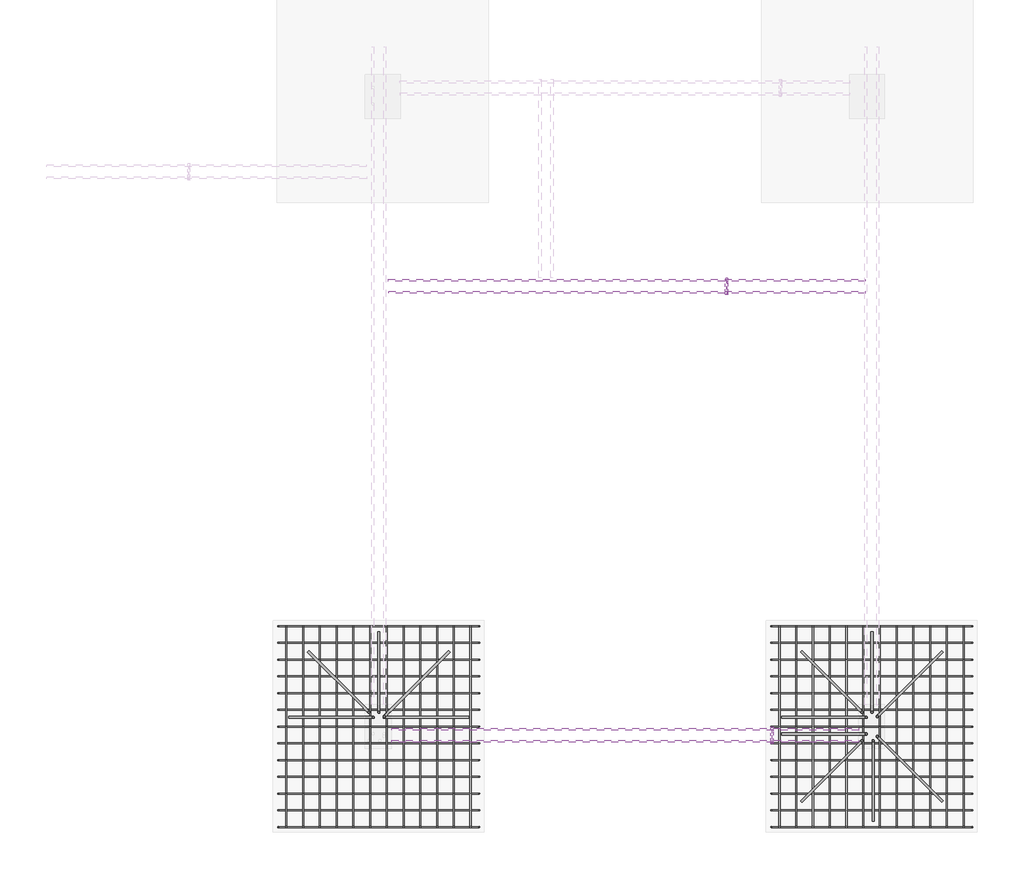
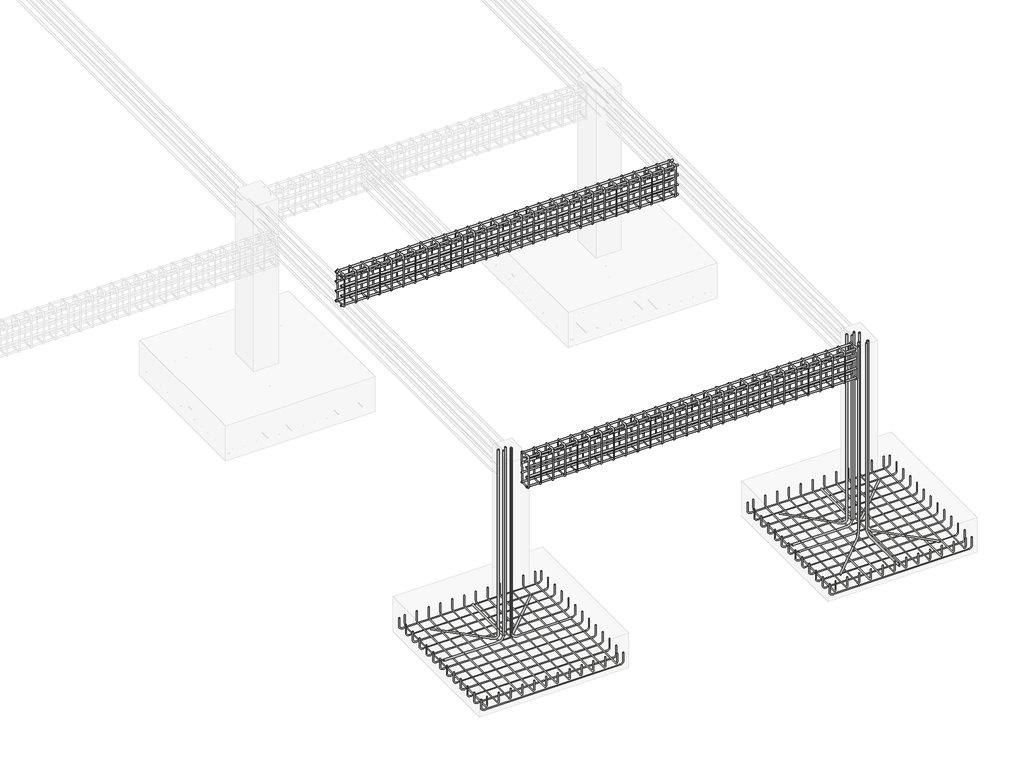
# One storey, part 3 of 10: 23 reinforcing bars.
"""IFC4 building model written with IfcOpenShell, lengths in millimetres."""

from ifc_helpers import new_model, si_unit, point, frame, origin, place, context, project, spatial, polyline, circle_curve, trimmed, segment, composite_curve, source, transform, mapped, element, save
from ifc_brep_helpers import swept_disk

model = new_model("IFC4")

# Units and contexts
model_context = context("Model", 3, world=origin())
ifc_project = project(units=[si_unit("LENGTHUNIT", "METRE", prefix="MILLI")], contexts=[model_context])

# Site, building, storey
site = spatial("IfcSite", under=ifc_project)
building = spatial("IfcBuilding", under=site)
storey = spatial("IfcBuildingStorey", under=building, Elevation=-2133.6)

# Reinforcing bars
placement = place(None, origin())
reinforcing_bar_shape = source(origin(), model_context, "Body", "SolidModel", [
    swept_disk(composite_curve([segment(polyline([(4240.1835638, -3095.8780823, -2393.6), (4240.1835638, -3095.8780823, -2504.1)]), True, "CONTINUOUS"), segment(trimmed(circle_curve(frame((4205.4335638, -3095.8780823, -2504.1), z_axis=(0.0, 1.0, 0.0), x_axis=(34.75, 0.0, 0.0)), 34.75), [point((4240.1835638, -3095.8780823, -2504.1))], [point((4205.4335638, -3095.8780823, -2538.85))], True, "CARTESIAN"), True, "CONTINUOUS"), segment(polyline([(4205.4335638, -3095.8780823, -2538.85), (2535.6335638, -3095.8780823, -2538.85)]), True, "CONTINUOUS"), segment(trimmed(circle_curve(frame((2535.6335638, -3095.8780823, -2504.1), z_axis=(0.0, 1.0, 0.0), x_axis=(0.0, 0.0, -34.75)), 34.75), [point((2535.6335638, -3095.8780823, -2538.85))], [point((2500.8835638, -3095.8780823, -2504.1))], True, "CARTESIAN"), True, "CONTINUOUS"), segment(polyline([(2500.8835638, -3095.8780823, -2504.1), (2500.8835638, -3095.8780823, -2393.6)]), True, "CONTINUOUS")], self_intersect=False), 4.75),
])
element("IfcReinforcingBar", 1, at=placement, inside=storey, context=model_context, shape_type="MappedRepresentation", body=[
    mapped(reinforcing_bar_shape, transform((0.0, 0.0, 0.0), x_axis=(1.0, 0.0, 0.0), y_axis=(0.0, 1.0, 0.0), z_axis=(0.0, 0.0, 1.0))),
    mapped(reinforcing_bar_shape, transform((0.0, -144.9416667, 0.0), x_axis=(1.0, 0.0, 0.0), y_axis=(0.0, 1.0, 0.0), z_axis=(0.0, 0.0, 1.0))),
    mapped(reinforcing_bar_shape, transform((0.0, -289.8833333, 0.0), x_axis=(1.0, 0.0, 0.0), y_axis=(0.0, 1.0, 0.0), z_axis=(0.0, 0.0, 1.0))),
    mapped(reinforcing_bar_shape, transform((0.0, -434.825, 0.0), x_axis=(1.0, 0.0, 0.0), y_axis=(0.0, 1.0, 0.0), z_axis=(0.0, 0.0, 1.0))),
    mapped(reinforcing_bar_shape, transform((0.0, -579.7666667, 0.0), x_axis=(1.0, 0.0, 0.0), y_axis=(0.0, 1.0, 0.0), z_axis=(0.0, 0.0, 1.0))),
    mapped(reinforcing_bar_shape, transform((0.0, -724.7083333, 0.0), x_axis=(1.0, 0.0, 0.0), y_axis=(0.0, 1.0, 0.0), z_axis=(0.0, 0.0, 1.0))),
    mapped(reinforcing_bar_shape, transform((0.0, -869.65, 0.0), x_axis=(1.0, 0.0, 0.0), y_axis=(0.0, 1.0, 0.0), z_axis=(0.0, 0.0, 1.0))),
    mapped(reinforcing_bar_shape, transform((0.0, -1014.5916667, 0.0), x_axis=(1.0, 0.0, 0.0), y_axis=(0.0, 1.0, 0.0), z_axis=(0.0, 0.0, 1.0))),
    mapped(reinforcing_bar_shape, transform((0.0, -1159.5333333, 0.0), x_axis=(1.0, 0.0, 0.0), y_axis=(0.0, 1.0, 0.0), z_axis=(0.0, 0.0, 1.0))),
    mapped(reinforcing_bar_shape, transform((0.0, -1304.475, 0.0), x_axis=(1.0, 0.0, 0.0), y_axis=(0.0, 1.0, 0.0), z_axis=(0.0, 0.0, 1.0))),
    mapped(reinforcing_bar_shape, transform((0.0, -1449.4166667, 0.0), x_axis=(1.0, 0.0, 0.0), y_axis=(0.0, 1.0, 0.0), z_axis=(0.0, 0.0, 1.0))),
    mapped(reinforcing_bar_shape, transform((0.0, -1594.3583333, 0.0), x_axis=(1.0, 0.0, 0.0), y_axis=(0.0, 1.0, 0.0), z_axis=(0.0, 0.0, 1.0))),
    mapped(reinforcing_bar_shape, transform((0.0, -1739.3, 0.0), x_axis=(1.0, 0.0, 0.0), y_axis=(0.0, 1.0, 0.0), z_axis=(0.0, 0.0, 1.0))),
])
reinforcing_bar_2_shape = source(origin(), model_context, "Body", "SolidModel", [
    swept_disk(composite_curve([segment(polyline([(4165.2256133, -4835.1780823, -2379.223371), (4165.2256133, -4835.1780823, -2489.723371)]), True, "CONTINUOUS"), segment(trimmed(circle_curve(frame((4165.2256133, -4800.4280823, -2489.723371), z_axis=(1.0, 0.0, 0.0), x_axis=(0.0, -34.75, 0.0)), 34.75), [point((4165.2256133, -4835.1780823, -2489.723371))], [point((4165.2256133, -4800.4280823, -2524.473371))], True, "CARTESIAN"), True, "CONTINUOUS"), segment(polyline([(4165.2256133, -4800.4280823, -2524.473371), (4165.2256133, -3130.6280823, -2524.473371)]), True, "CONTINUOUS"), segment(trimmed(circle_curve(frame((4165.2256133, -3130.6280823, -2489.723371), z_axis=(1.0, 0.0, 0.0), x_axis=(0.0, 0.0, -34.75)), 34.75), [point((4165.2256133, -3130.6280823, -2524.473371))], [point((4165.2256133, -3095.8780823, -2489.723371))], True, "CARTESIAN"), True, "CONTINUOUS"), segment(polyline([(4165.2256133, -3095.8780823, -2489.723371), (4165.2256133, -3095.8780823, -2379.223371)]), True, "CONTINUOUS")], self_intersect=False), 4.75),
])
element("IfcReinforcingBar", 2, at=placement, inside=storey, context=model_context, shape_type="MappedRepresentation", body=[
    mapped(reinforcing_bar_2_shape, transform((0.0, 0.0, 0.0), x_axis=(1.0, 0.0, 0.0), y_axis=(0.0, 1.0, 0.0), z_axis=(0.0, 0.0, 1.0))),
    mapped(reinforcing_bar_2_shape, transform((-144.8323389, 0.0, 0.0), x_axis=(1.0, 0.0, 0.0), y_axis=(0.0, 1.0, 0.0), z_axis=(0.0, 0.0, 1.0))),
    mapped(reinforcing_bar_2_shape, transform((-289.6646779, 0.0, 0.0), x_axis=(1.0, 0.0, 0.0), y_axis=(0.0, 1.0, 0.0), z_axis=(0.0, 0.0, 1.0))),
    mapped(reinforcing_bar_2_shape, transform((-434.4970168, 0.0, 0.0), x_axis=(1.0, 0.0, 0.0), y_axis=(0.0, 1.0, 0.0), z_axis=(0.0, 0.0, 1.0))),
    mapped(reinforcing_bar_2_shape, transform((-579.3293558, 0.0, 0.0), x_axis=(1.0, 0.0, 0.0), y_axis=(0.0, 1.0, 0.0), z_axis=(0.0, 0.0, 1.0))),
    mapped(reinforcing_bar_2_shape, transform((-724.1616947, 0.0, 0.0), x_axis=(1.0, 0.0, 0.0), y_axis=(0.0, 1.0, 0.0), z_axis=(0.0, 0.0, 1.0))),
    mapped(reinforcing_bar_2_shape, transform((-868.9940337, 0.0, 0.0), x_axis=(1.0, 0.0, 0.0), y_axis=(0.0, 1.0, 0.0), z_axis=(0.0, 0.0, 1.0))),
    mapped(reinforcing_bar_2_shape, transform((-1013.8263726, 0.0, 0.0), x_axis=(1.0, 0.0, 0.0), y_axis=(0.0, 1.0, 0.0), z_axis=(0.0, 0.0, 1.0))),
    mapped(reinforcing_bar_2_shape, transform((-1158.6587116, 0.0, 0.0), x_axis=(1.0, 0.0, 0.0), y_axis=(0.0, 1.0, 0.0), z_axis=(0.0, 0.0, 1.0))),
    mapped(reinforcing_bar_2_shape, transform((-1303.4910505, 0.0, 0.0), x_axis=(1.0, 0.0, 0.0), y_axis=(0.0, 1.0, 0.0), z_axis=(0.0, 0.0, 1.0))),
    mapped(reinforcing_bar_2_shape, transform((-1448.3233895, 0.0, 0.0), x_axis=(1.0, 0.0, 0.0), y_axis=(0.0, 1.0, 0.0), z_axis=(0.0, 0.0, 1.0))),
    mapped(reinforcing_bar_2_shape, transform((-1593.1557284, 0.0, 0.0), x_axis=(1.0, 0.0, 0.0), y_axis=(0.0, 1.0, 0.0), z_axis=(0.0, 0.0, 1.0))),
])
reinforcing_bar_3_shape = source(origin(), model_context, "Body", "SolidModel", [
    swept_disk(composite_curve([segment(polyline([(8507.3835638, -3095.8780823, -2393.6), (8507.3835638, -3095.8780823, -2504.1)]), True, "CONTINUOUS"), segment(trimmed(circle_curve(frame((8472.6335638, -3095.8780823, -2504.1), z_axis=(0.0, 1.0, 0.0), x_axis=(34.75, 0.0, 0.0)), 34.75), [point((8507.3835638, -3095.8780823, -2504.1))], [point((8472.6335638, -3095.8780823, -2538.85))], True, "CARTESIAN"), True, "CONTINUOUS"), segment(polyline([(8472.6335638, -3095.8780823, -2538.85), (6802.8335638, -3095.8780823, -2538.85)]), True, "CONTINUOUS"), segment(trimmed(circle_curve(frame((6802.8335638, -3095.8780823, -2504.1), z_axis=(0.0, 1.0, 0.0), x_axis=(0.0, 0.0, -34.75)), 34.75), [point((6802.8335638, -3095.8780823, -2538.85))], [point((6768.0835638, -3095.8780823, -2504.1))], True, "CARTESIAN"), True, "CONTINUOUS"), segment(polyline([(6768.0835638, -3095.8780823, -2504.1), (6768.0835638, -3095.8780823, -2393.6)]), True, "CONTINUOUS")], self_intersect=False), 4.75),
])
element("IfcReinforcingBar", 3, at=placement, inside=storey, context=model_context, shape_type="MappedRepresentation", body=[
    mapped(reinforcing_bar_3_shape, transform((0.0, 0.0, 0.0), x_axis=(1.0, 0.0, 0.0), y_axis=(0.0, 1.0, 0.0), z_axis=(0.0, 0.0, 1.0))),
    mapped(reinforcing_bar_3_shape, transform((0.0, -144.9416667, 0.0), x_axis=(1.0, 0.0, 0.0), y_axis=(0.0, 1.0, 0.0), z_axis=(0.0, 0.0, 1.0))),
    mapped(reinforcing_bar_3_shape, transform((0.0, -289.8833333, 0.0), x_axis=(1.0, 0.0, 0.0), y_axis=(0.0, 1.0, 0.0), z_axis=(0.0, 0.0, 1.0))),
    mapped(reinforcing_bar_3_shape, transform((0.0, -434.825, 0.0), x_axis=(1.0, 0.0, 0.0), y_axis=(0.0, 1.0, 0.0), z_axis=(0.0, 0.0, 1.0))),
    mapped(reinforcing_bar_3_shape, transform((0.0, -579.7666667, 0.0), x_axis=(1.0, 0.0, 0.0), y_axis=(0.0, 1.0, 0.0), z_axis=(0.0, 0.0, 1.0))),
    mapped(reinforcing_bar_3_shape, transform((0.0, -724.7083333, 0.0), x_axis=(1.0, 0.0, 0.0), y_axis=(0.0, 1.0, 0.0), z_axis=(0.0, 0.0, 1.0))),
    mapped(reinforcing_bar_3_shape, transform((0.0, -869.65, 0.0), x_axis=(1.0, 0.0, 0.0), y_axis=(0.0, 1.0, 0.0), z_axis=(0.0, 0.0, 1.0))),
    mapped(reinforcing_bar_3_shape, transform((0.0, -1014.5916667, 0.0), x_axis=(1.0, 0.0, 0.0), y_axis=(0.0, 1.0, 0.0), z_axis=(0.0, 0.0, 1.0))),
    mapped(reinforcing_bar_3_shape, transform((0.0, -1159.5333333, 0.0), x_axis=(1.0, 0.0, 0.0), y_axis=(0.0, 1.0, 0.0), z_axis=(0.0, 0.0, 1.0))),
    mapped(reinforcing_bar_3_shape, transform((0.0, -1304.475, 0.0), x_axis=(1.0, 0.0, 0.0), y_axis=(0.0, 1.0, 0.0), z_axis=(0.0, 0.0, 1.0))),
    mapped(reinforcing_bar_3_shape, transform((0.0, -1449.4166667, 0.0), x_axis=(1.0, 0.0, 0.0), y_axis=(0.0, 1.0, 0.0), z_axis=(0.0, 0.0, 1.0))),
    mapped(reinforcing_bar_3_shape, transform((0.0, -1594.3583333, 0.0), x_axis=(1.0, 0.0, 0.0), y_axis=(0.0, 1.0, 0.0), z_axis=(0.0, 0.0, 1.0))),
    mapped(reinforcing_bar_3_shape, transform((0.0, -1739.3, 0.0), x_axis=(1.0, 0.0, 0.0), y_axis=(0.0, 1.0, 0.0), z_axis=(0.0, 0.0, 1.0))),
])
reinforcing_bar_4_shape = source(origin(), model_context, "Body", "SolidModel", [
    swept_disk(composite_curve([segment(polyline([(8432.4256133, -4835.1780823, -2379.223371), (8432.4256133, -4835.1780823, -2489.723371)]), True, "CONTINUOUS"), segment(trimmed(circle_curve(frame((8432.4256133, -4800.4280823, -2489.723371), z_axis=(1.0, 0.0, 0.0), x_axis=(0.0, -34.75, 0.0)), 34.75), [point((8432.4256133, -4835.1780823, -2489.723371))], [point((8432.4256133, -4800.4280823, -2524.473371))], True, "CARTESIAN"), True, "CONTINUOUS"), segment(polyline([(8432.4256133, -4800.4280823, -2524.473371), (8432.4256133, -3130.6280823, -2524.473371)]), True, "CONTINUOUS"), segment(trimmed(circle_curve(frame((8432.4256133, -3130.6280823, -2489.723371), z_axis=(1.0, 0.0, 0.0), x_axis=(0.0, 0.0, -34.75)), 34.75), [point((8432.4256133, -3130.6280823, -2524.473371))], [point((8432.4256133, -3095.8780823, -2489.723371))], True, "CARTESIAN"), True, "CONTINUOUS"), segment(polyline([(8432.4256133, -3095.8780823, -2489.723371), (8432.4256133, -3095.8780823, -2379.223371)]), True, "CONTINUOUS")], self_intersect=False), 4.75),
])
element("IfcReinforcingBar", 4, at=placement, inside=storey, context=model_context, shape_type="MappedRepresentation", body=[
    mapped(reinforcing_bar_4_shape, transform((0.0, 0.0, 0.0), x_axis=(1.0, 0.0, 0.0), y_axis=(0.0, 1.0, 0.0), z_axis=(0.0, 0.0, 1.0))),
    mapped(reinforcing_bar_4_shape, transform((-144.8323389, 0.0, 0.0), x_axis=(1.0, 0.0, 0.0), y_axis=(0.0, 1.0, 0.0), z_axis=(0.0, 0.0, 1.0))),
    mapped(reinforcing_bar_4_shape, transform((-289.6646779, 0.0, 0.0), x_axis=(1.0, 0.0, 0.0), y_axis=(0.0, 1.0, 0.0), z_axis=(0.0, 0.0, 1.0))),
    mapped(reinforcing_bar_4_shape, transform((-434.4970168, 0.0, 0.0), x_axis=(1.0, 0.0, 0.0), y_axis=(0.0, 1.0, 0.0), z_axis=(0.0, 0.0, 1.0))),
    mapped(reinforcing_bar_4_shape, transform((-579.3293558, 0.0, 0.0), x_axis=(1.0, 0.0, 0.0), y_axis=(0.0, 1.0, 0.0), z_axis=(0.0, 0.0, 1.0))),
    mapped(reinforcing_bar_4_shape, transform((-724.1616947, 0.0, 0.0), x_axis=(1.0, 0.0, 0.0), y_axis=(0.0, 1.0, 0.0), z_axis=(0.0, 0.0, 1.0))),
    mapped(reinforcing_bar_4_shape, transform((-868.9940337, 0.0, 0.0), x_axis=(1.0, 0.0, 0.0), y_axis=(0.0, 1.0, 0.0), z_axis=(0.0, 0.0, 1.0))),
    mapped(reinforcing_bar_4_shape, transform((-1013.8263726, 0.0, 0.0), x_axis=(1.0, 0.0, 0.0), y_axis=(0.0, 1.0, 0.0), z_axis=(0.0, 0.0, 1.0))),
    mapped(reinforcing_bar_4_shape, transform((-1158.6587116, 0.0, 0.0), x_axis=(1.0, 0.0, 0.0), y_axis=(0.0, 1.0, 0.0), z_axis=(0.0, 0.0, 1.0))),
    mapped(reinforcing_bar_4_shape, transform((-1303.4910505, 0.0, 0.0), x_axis=(1.0, 0.0, 0.0), y_axis=(0.0, 1.0, 0.0), z_axis=(0.0, 0.0, 1.0))),
    mapped(reinforcing_bar_4_shape, transform((-1448.3233895, 0.0, 0.0), x_axis=(1.0, 0.0, 0.0), y_axis=(0.0, 1.0, 0.0), z_axis=(0.0, 0.0, 1.0))),
    mapped(reinforcing_bar_4_shape, transform((-1593.1557284, 0.0, 0.0), x_axis=(1.0, 0.0, 0.0), y_axis=(0.0, 1.0, 0.0), z_axis=(0.0, 0.0, 1.0))),
])
element("IfcReinforcingBar", 5, at=placement, inside=storey, context=model_context, shape_type="SolidModel", body=[
    swept_disk(composite_curve([segment(polyline([(7552.4335638, -3841.2447039, -40.0), (7552.4335638, -3841.2447039, -2426.55)]), True, "CONTINUOUS"), segment(trimmed(circle_curve(frame((7505.0220542, -3793.8331942, -2426.55), z_axis=(0.7071067811865519, 0.7071067811865431, 0.0), x_axis=(47.4115096000005, -47.4115096999999, 0.0)), 67.05), [point((7552.4335638, -3841.2447039, -2426.55))], [point((7505.0220542, -3793.8331942, -2493.6))], True, "CARTESIAN"), True, "CONTINUOUS"), segment(polyline([(7505.0220542, -3793.8331942, -2493.6), (7028.0116308, -3316.8227708, -2493.6)]), True, "CONTINUOUS")], self_intersect=False), 9.55),
])
element("IfcReinforcingBar", 6, at=placement, inside=storey, context=model_context, shape_type="SolidModel", body=[
    swept_disk(composite_curve([segment(polyline([(7686.0335638, -3879.3447039, -40.0), (7686.0335638, -3879.3447039, -2426.55)]), True, "CONTINUOUS"), segment(trimmed(circle_curve(frame((7733.4450735, -3831.9331942, -2426.55), z_axis=(0.7071067811865519, -0.7071067811865431, 0.0), x_axis=(-47.41150970000035, -47.4115096999999, 0.0)), 67.05), [point((7686.0335638, -3879.3447039, -2426.55))], [point((7733.4450735, -3831.9331942, -2493.6))], True, "CARTESIAN"), True, "CONTINUOUS"), segment(polyline([(7733.4450735, -3831.9331942, -2493.6), (8248.5554969, -3316.8227708, -2493.6)]), True, "CONTINUOUS")], self_intersect=False), 9.55),
])
element("IfcReinforcingBar", 7, at=placement, inside=storey, context=model_context, shape_type="SolidModel", body=[
    swept_disk(composite_curve([segment(polyline([(7552.4335638, -4089.8114607, -40.0), (7552.4335638, -4089.8114607, -2426.55)]), True, "CONTINUOUS"), segment(trimmed(circle_curve(frame((7505.0220542, -4137.2229704, -2426.55), z_axis=(-0.7071067811865519, 0.7071067811865431, 0.0), x_axis=(47.4115096000005, 47.4115096999999, 0.0)), 67.05), [point((7552.4335638, -4089.8114607, -2426.55))], [point((7505.0220542, -4137.2229704, -2493.6))], True, "CARTESIAN"), True, "CONTINUOUS"), segment(polyline([(7505.0220542, -4137.2229704, -2493.6), (7028.0116308, -4614.2333938, -2493.6)]), True, "CONTINUOUS")], self_intersect=False), 9.55),
])
element("IfcReinforcingBar", 8, at=placement, inside=storey, context=model_context, shape_type="SolidModel", body=[
    swept_disk(composite_curve([segment(polyline([(7686.0335638, -4051.7114607, -40.0), (7686.0335638, -4051.7114607, -2426.55)]), True, "CONTINUOUS"), segment(trimmed(circle_curve(frame((7733.4450735, -4099.1229704, -2426.55), z_axis=(-0.7071067811865519, -0.7071067811865431, 0.0), x_axis=(-47.41150970000035, 47.4115096999999, 0.0)), 67.05), [point((7686.0335638, -4051.7114607, -2426.55))], [point((7733.4450735, -4099.1229704, -2493.6))], True, "CARTESIAN"), True, "CONTINUOUS"), segment(polyline([(7733.4450735, -4099.1229704, -2493.6), (8248.5554969, -4614.2333938, -2493.6)]), True, "CONTINUOUS")], self_intersect=False), 9.55),
])
element("IfcReinforcingBar", 9, at=placement, inside=storey, context=model_context, shape_type="SolidModel", body=[
    swept_disk(composite_curve([segment(polyline([(7639.4194855, -3841.2447039, -40.0), (7639.4194855, -3841.2447039, -2426.55)]), True, "CONTINUOUS"), segment(trimmed(circle_curve(frame((7639.4194855, -3774.1947039, -2426.55), z_axis=(1.0, 0.0, 0.0), x_axis=(0.0, -67.04999999999973, 0.0)), 67.05), [point((7639.4194855, -3841.2447039, -2426.55))], [point((7639.4194855, -3774.1947039, -2493.6))], True, "CARTESIAN"), True, "CONTINUOUS"), segment(polyline([(7639.4194855, -3774.1947039, -2493.6), (7639.4194855, -3146.9447039, -2493.6)]), True, "CONTINUOUS")], self_intersect=False), 9.55),
])
element("IfcReinforcingBar", 10, at=placement, inside=storey, context=model_context, shape_type="SolidModel", body=[
    swept_disk(composite_curve([segment(polyline([(7649.4194855, -4089.8114607, -40.0), (7649.4194855, -4089.8114607, -2426.55)]), True, "CONTINUOUS"), segment(trimmed(circle_curve(frame((7649.4194855, -4156.8614607, -2426.55), z_axis=(-1.0, 0.0, 0.0), x_axis=(0.0, 67.04999999999973, 0.0)), 67.05), [point((7649.4194855, -4089.8114607, -2426.55))], [point((7649.4194855, -4156.8614607, -2493.6))], True, "CARTESIAN"), True, "CONTINUOUS"), segment(polyline([(7649.4194855, -4156.8614607, -2493.6), (7649.4194855, -4784.1114607, -2493.6)]), True, "CONTINUOUS")], self_intersect=False), 9.55),
])
element("IfcReinforcingBar", 11, at=placement, inside=storey, context=model_context, shape_type="SolidModel", body=[
    swept_disk(composite_curve([segment(polyline([(7590.5335638, -3886.2447039, -40.0), (7590.5335638, -3886.2447039, -2426.55)]), True, "CONTINUOUS"), segment(trimmed(circle_curve(frame((7523.4835638, -3886.2447039, -2426.55), z_axis=(0.0, 1.0, 0.0), x_axis=(67.04999999999927, 0.0, 0.0)), 67.05), [point((7590.5335638, -3886.2447039, -2426.55))], [point((7523.4835638, -3886.2447039, -2493.6))], True, "CARTESIAN"), True, "CONTINUOUS"), segment(polyline([(7523.4835638, -3886.2447039, -2493.6), (6858.1335638, -3886.2447039, -2493.6)]), True, "CONTINUOUS")], self_intersect=False), 9.55),
])
element("IfcReinforcingBar", 12, at=placement, inside=storey, context=model_context, shape_type="SolidModel", body=[
    swept_disk(composite_curve([segment(polyline([(7590.5335638, -4029.5829002, -40.0), (7590.5335638, -4029.5829002, -2426.55)]), True, "CONTINUOUS"), segment(trimmed(circle_curve(frame((7523.4835638, -4029.5829002, -2426.55), z_axis=(0.0, 1.0, 0.0), x_axis=(67.04999999999927, 0.0, 0.0)), 67.05), [point((7590.5335638, -4029.5829002, -2426.55))], [point((7523.4835638, -4029.5829002, -2493.6))], True, "CARTESIAN"), True, "CONTINUOUS"), segment(polyline([(7523.4835638, -4029.5829002, -2493.6), (6858.1335638, -4029.5829002, -2493.6)]), True, "CONTINUOUS")], self_intersect=False), 9.55),
])
element("IfcReinforcingBar", 13, at=placement, inside=storey, context=model_context, shape_type="SolidModel", body=[
    swept_disk(composite_curve([segment(polyline([(3285.2335638, -3841.2447039, -40.0), (3285.2335638, -3841.2447039, -2426.55)]), True, "CONTINUOUS"), segment(trimmed(circle_curve(frame((3237.8220542, -3793.8331942, -2426.55), z_axis=(0.7071067811865519, 0.7071067811865431, 0.0), x_axis=(47.411509600000045, -47.4115096999999, 0.0)), 67.05), [point((3285.2335638, -3841.2447039, -2426.55))], [point((3237.8220542, -3793.8331942, -2493.6))], True, "CARTESIAN"), True, "CONTINUOUS"), segment(polyline([(3237.8220542, -3793.8331942, -2493.6), (2760.8116308, -3316.8227708, -2493.6)]), True, "CONTINUOUS")], self_intersect=False), 9.55),
])
element("IfcReinforcingBar", 14, at=placement, inside=storey, context=model_context, shape_type="SolidModel", body=[
    swept_disk(composite_curve([segment(polyline([(3418.8335638, -3879.3447039, -40.0), (3418.8335638, -3879.3447039, -2426.55)]), True, "CONTINUOUS"), segment(trimmed(circle_curve(frame((3466.2450735, -3831.9331942, -2426.55), z_axis=(0.7071067811865519, -0.7071067811865431, 0.0), x_axis=(-47.41150970000035, -47.4115096999999, 0.0)), 67.05), [point((3418.8335638, -3879.3447039, -2426.55))], [point((3466.2450735, -3831.9331942, -2493.6))], True, "CARTESIAN"), True, "CONTINUOUS"), segment(polyline([(3466.2450735, -3831.9331942, -2493.6), (3981.3554969, -3316.8227708, -2493.6)]), True, "CONTINUOUS")], self_intersect=False), 9.55),
])
element("IfcReinforcingBar", 15, at=placement, inside=storey, context=model_context, shape_type="SolidModel", body=[
    swept_disk(composite_curve([segment(polyline([(3372.2194855, -3841.2447039, -40.0), (3372.2194855, -3841.2447039, -2426.55)]), True, "CONTINUOUS"), segment(trimmed(circle_curve(frame((3372.2194855, -3774.1947039, -2426.55), z_axis=(1.0, 0.0, 0.0), x_axis=(0.0, -67.04999999999973, 0.0)), 67.05), [point((3372.2194855, -3841.2447039, -2426.55))], [point((3372.2194855, -3774.1947039, -2493.6))], True, "CARTESIAN"), True, "CONTINUOUS"), segment(polyline([(3372.2194855, -3774.1947039, -2493.6), (3372.2194855, -3146.9447039, -2493.6)]), True, "CONTINUOUS")], self_intersect=False), 9.55),
])
element("IfcReinforcingBar", 16, at=placement, inside=storey, context=model_context, shape_type="SolidModel", body=[
    swept_disk(composite_curve([segment(polyline([(3323.3335638, -3886.2447039, -40.0), (3323.3335638, -3886.2447039, -2426.55)]), True, "CONTINUOUS"), segment(trimmed(circle_curve(frame((3256.2835638, -3886.2447039, -2426.55), z_axis=(0.0, 1.0, 0.0), x_axis=(67.04999999999973, 0.0, 0.0)), 67.05), [point((3323.3335638, -3886.2447039, -2426.55))], [point((3256.2835638, -3886.2447039, -2493.6))], True, "CARTESIAN"), True, "CONTINUOUS"), segment(polyline([(3256.2835638, -3886.2447039, -2493.6), (2590.9335638, -3886.2447039, -2493.6)]), True, "CONTINUOUS")], self_intersect=False), 9.55),
])
element("IfcReinforcingBar", 17, at=placement, inside=storey, context=model_context, shape_type="SolidModel", body=[
    swept_disk(composite_curve([segment(polyline([(3418.8335638, -3886.2447039, -40.0), (3418.8335638, -3886.2447039, -2426.55)]), True, "CONTINUOUS"), segment(trimmed(circle_curve(frame((3485.8835638, -3886.2447039, -2426.55), z_axis=(0.0, -1.0, 0.0), x_axis=(-67.05000000000018, 0.0, 0.0)), 67.05), [point((3418.8335638, -3886.2447039, -2426.55))], [point((3485.8835638, -3886.2447039, -2493.6))], True, "CARTESIAN"), True, "CONTINUOUS"), segment(polyline([(3485.8835638, -3886.2447039, -2493.6), (4151.2335638, -3886.2447039, -2493.6)]), True, "CONTINUOUS")], self_intersect=False), 9.55),
])
reinforcing_bar_5_shape = source(origin(), model_context, "Body", "SolidModel", [
    swept_disk(composite_curve([segment(polyline([(3502.9475179, -4011.6213007, -109.4049959), (3502.9475179, -4069.0271895, -51.9991072)]), True, "CONTINUOUS"), segment(trimmed(circle_curve(frame((3502.9475179, -4086.5280823, -69.5), z_axis=(1.0, 0.0, 0.0), x_axis=(0.0, 17.500892799999747, 17.500892800000003)), 24.75), [point((3502.9475179, -4069.0271895, -51.9991072))], [point((3502.9475179, -4111.2780823, -69.5))], True, "CARTESIAN"), True, "CONTINUOUS"), segment(polyline([(3502.9475179, -4111.2780823, -69.5), (3502.9475179, -4111.2780823, -430.5)]), True, "CONTINUOUS"), segment(trimmed(circle_curve(frame((3502.9475179, -4086.5280823, -430.5), z_axis=(1.0, 0.0, 0.0), x_axis=(0.0, -24.750000000000455, 0.0)), 24.75), [point((3502.9475179, -4111.2780823, -430.5))], [point((3502.9475179, -4086.5280823, -455.25))], True, "CARTESIAN"), True, "CONTINUOUS"), segment(polyline([(3502.9475179, -4086.5280823, -455.25), (3502.9475179, -3996.9280823, -455.25)]), True, "CONTINUOUS"), segment(trimmed(circle_curve(frame((3502.3748941, -3996.9280823, -430.5066251), z_axis=(0.9997323196529888, 0.0, 0.02313631434032496), x_axis=(0.5726238000002013, 0.0, -24.743374899999992)), 24.75), [point((3502.9475179, -3996.9280823, -455.25))], [point((3502.3748941, -3972.1780823, -430.5066251))], True, "CARTESIAN"), True, "CONTINUOUS"), segment(polyline([(3502.3748941, -3972.1780823, -430.5066251), (3494.0201417, -3972.1780823, -69.4933749)]), True, "CONTINUOUS"), segment(trimmed(circle_curve(frame((3494.0201417, -3996.9280823, -69.4933749), z_axis=(0.9997323196529888, 0.0, 0.02313631434032496), x_axis=(0.0, 24.75, 0.0)), 24.75), [point((3494.0201417, -3972.1780823, -69.4933749))], [point((3493.4475179, -3996.9280823, -44.75))], True, "CARTESIAN"), True, "CONTINUOUS"), segment(polyline([(3493.4475179, -3996.9280823, -44.75), (3493.4475179, -4086.5280823, -44.75)]), True, "CONTINUOUS"), segment(trimmed(circle_curve(frame((3493.4475179, -4086.5280823, -69.5), z_axis=(1.0, 0.0, 0.0), x_axis=(0.0, 0.0, 24.75)), 24.75), [point((3493.4475179, -4086.5280823, -44.75))], [point((3493.4475179, -4104.0289751, -87.0008928))], True, "CARTESIAN"), True, "CONTINUOUS"), segment(polyline([(3493.4475179, -4104.0289751, -87.0008928), (3493.4475179, -4046.6230864, -144.4067815)]), True, "CONTINUOUS")], self_intersect=False), 4.75),
])
element("IfcReinforcingBar", 18, at=placement, inside=storey, context=model_context, shape_type="MappedRepresentation", body=[
    mapped(reinforcing_bar_5_shape, transform((0.0, 0.0, 0.0), x_axis=(1.0, 0.0, 0.0), y_axis=(0.0, 1.0, 0.0), z_axis=(0.0, 0.0, 1.0))),
    mapped(reinforcing_bar_5_shape, transform((148.9068906, 0.0, 0.0), x_axis=(1.0, 0.0, 0.0), y_axis=(0.0, 1.0, 0.0), z_axis=(0.0, 0.0, 1.0))),
    mapped(reinforcing_bar_5_shape, transform((297.8137812, 0.0, 0.0), x_axis=(1.0, 0.0, 0.0), y_axis=(0.0, 1.0, 0.0), z_axis=(0.0, 0.0, 1.0))),
    mapped(reinforcing_bar_5_shape, transform((446.7206718, 0.0, 0.0), x_axis=(1.0, 0.0, 0.0), y_axis=(0.0, 1.0, 0.0), z_axis=(0.0, 0.0, 1.0))),
    mapped(reinforcing_bar_5_shape, transform((595.6275624, 0.0, 0.0), x_axis=(1.0, 0.0, 0.0), y_axis=(0.0, 1.0, 0.0), z_axis=(0.0, 0.0, 1.0))),
    mapped(reinforcing_bar_5_shape, transform((744.5344529, 0.0, 0.0), x_axis=(1.0, 0.0, 0.0), y_axis=(0.0, 1.0, 0.0), z_axis=(0.0, 0.0, 1.0))),
    mapped(reinforcing_bar_5_shape, transform((893.4413435, 0.0, 0.0), x_axis=(1.0, 0.0, 0.0), y_axis=(0.0, 1.0, 0.0), z_axis=(0.0, 0.0, 1.0))),
    mapped(reinforcing_bar_5_shape, transform((1042.3482341, 0.0, 0.0), x_axis=(1.0, 0.0, 0.0), y_axis=(0.0, 1.0, 0.0), z_axis=(0.0, 0.0, 1.0))),
    mapped(reinforcing_bar_5_shape, transform((1191.2551247, 0.0, 0.0), x_axis=(1.0, 0.0, 0.0), y_axis=(0.0, 1.0, 0.0), z_axis=(0.0, 0.0, 1.0))),
    mapped(reinforcing_bar_5_shape, transform((1340.1620153, 0.0, 0.0), x_axis=(1.0, 0.0, 0.0), y_axis=(0.0, 1.0, 0.0), z_axis=(0.0, 0.0, 1.0))),
    mapped(reinforcing_bar_5_shape, transform((1489.0689059, 0.0, 0.0), x_axis=(1.0, 0.0, 0.0), y_axis=(0.0, 1.0, 0.0), z_axis=(0.0, 0.0, 1.0))),
    mapped(reinforcing_bar_5_shape, transform((1637.9757965, 0.0, 0.0), x_axis=(1.0, 0.0, 0.0), y_axis=(0.0, 1.0, 0.0), z_axis=(0.0, 0.0, 1.0))),
    mapped(reinforcing_bar_5_shape, transform((1786.8826871, 0.0, 0.0), x_axis=(1.0, 0.0, 0.0), y_axis=(0.0, 1.0, 0.0), z_axis=(0.0, 0.0, 1.0))),
    mapped(reinforcing_bar_5_shape, transform((1935.7895777, 0.0, 0.0), x_axis=(1.0, 0.0, 0.0), y_axis=(0.0, 1.0, 0.0), z_axis=(0.0, 0.0, 1.0))),
    mapped(reinforcing_bar_5_shape, transform((2084.6964683, 0.0, 0.0), x_axis=(1.0, 0.0, 0.0), y_axis=(0.0, 1.0, 0.0), z_axis=(0.0, 0.0, 1.0))),
    mapped(reinforcing_bar_5_shape, transform((2233.6033588, 0.0, 0.0), x_axis=(1.0, 0.0, 0.0), y_axis=(0.0, 1.0, 0.0), z_axis=(0.0, 0.0, 1.0))),
    mapped(reinforcing_bar_5_shape, transform((2382.5102494, 0.0, 0.0), x_axis=(1.0, 0.0, 0.0), y_axis=(0.0, 1.0, 0.0), z_axis=(0.0, 0.0, 1.0))),
    mapped(reinforcing_bar_5_shape, transform((2531.41714, 0.0, 0.0), x_axis=(1.0, 0.0, 0.0), y_axis=(0.0, 1.0, 0.0), z_axis=(0.0, 0.0, 1.0))),
    mapped(reinforcing_bar_5_shape, transform((2680.3240306, 0.0, 0.0), x_axis=(1.0, 0.0, 0.0), y_axis=(0.0, 1.0, 0.0), z_axis=(0.0, 0.0, 1.0))),
    mapped(reinforcing_bar_5_shape, transform((2829.2309212, 0.0, 0.0), x_axis=(1.0, 0.0, 0.0), y_axis=(0.0, 1.0, 0.0), z_axis=(0.0, 0.0, 1.0))),
    mapped(reinforcing_bar_5_shape, transform((2978.1378118, 0.0, 0.0), x_axis=(1.0, 0.0, 0.0), y_axis=(0.0, 1.0, 0.0), z_axis=(0.0, 0.0, 1.0))),
    mapped(reinforcing_bar_5_shape, transform((3127.0447024, 0.0, 0.0), x_axis=(1.0, 0.0, 0.0), y_axis=(0.0, 1.0, 0.0), z_axis=(0.0, 0.0, 1.0))),
    mapped(reinforcing_bar_5_shape, transform((3275.951593, 0.0, 0.0), x_axis=(1.0, 0.0, 0.0), y_axis=(0.0, 1.0, 0.0), z_axis=(0.0, 0.0, 1.0))),
    mapped(reinforcing_bar_5_shape, transform((3424.8584836, 0.0, 0.0), x_axis=(1.0, 0.0, 0.0), y_axis=(0.0, 1.0, 0.0), z_axis=(0.0, 0.0, 1.0))),
    mapped(reinforcing_bar_5_shape, transform((3573.7653741, 0.0, 0.0), x_axis=(1.0, 0.0, 0.0), y_axis=(0.0, 1.0, 0.0), z_axis=(0.0, 0.0, 1.0))),
    mapped(reinforcing_bar_5_shape, transform((3722.6722647, 0.0, 0.0), x_axis=(1.0, 0.0, 0.0), y_axis=(0.0, 1.0, 0.0), z_axis=(0.0, 0.0, 1.0))),
    mapped(reinforcing_bar_5_shape, transform((3871.5791553, 0.0, 0.0), x_axis=(1.0, 0.0, 0.0), y_axis=(0.0, 1.0, 0.0), z_axis=(0.0, 0.0, 1.0))),
    mapped(reinforcing_bar_5_shape, transform((4020.4860459, 0.0, 0.0), x_axis=(1.0, 0.0, 0.0), y_axis=(0.0, 1.0, 0.0), z_axis=(0.0, 0.0, 1.0))),
])
reinforcing_bar_6_shape = source(origin(), model_context, "Body", "SolidModel", [
    swept_disk(composite_curve([segment(polyline([(3483.3103419, -4093.9173481, -62.1107341), (7526.2572451, -4093.9173481, -62.1107341)]), True, "CONTINUOUS")], self_intersect=False), 9.55),
])
element("IfcReinforcingBar", 19, at=placement, inside=storey, context=model_context, shape_type="MappedRepresentation", body=[
    mapped(reinforcing_bar_6_shape, transform((0.0, 0.0, 0.0), x_axis=(1.0, 0.0, 0.0), y_axis=(0.0, 1.0, 0.0), z_axis=(0.0, 0.0, 1.0))),
    mapped(reinforcing_bar_6_shape, transform((0.0, 0.0, -125.2595106), x_axis=(1.0, 0.0, 0.0), y_axis=(0.0, 1.0, 0.0), z_axis=(0.0, 0.0, 1.0))),
    mapped(reinforcing_bar_6_shape, transform((0.0, 0.0, -250.5190212), x_axis=(1.0, 0.0, 0.0), y_axis=(0.0, 1.0, 0.0), z_axis=(0.0, 0.0, 1.0))),
    mapped(reinforcing_bar_6_shape, transform((0.0, 0.0, -375.7785317), x_axis=(1.0, 0.0, 0.0), y_axis=(0.0, 1.0, 0.0), z_axis=(0.0, 0.0, 1.0))),
])
reinforcing_bar_7_shape = source(origin(), model_context, "Body", "SolidModel", [
    swept_disk(composite_curve([segment(polyline([(3483.5768331, -3989.5388164, -62.1107341), (7524.875895, -3989.5388164, -62.1107341)]), True, "CONTINUOUS")], self_intersect=False), 9.55),
])
element("IfcReinforcingBar", 20, at=placement, inside=storey, context=model_context, shape_type="MappedRepresentation", body=[
    mapped(reinforcing_bar_7_shape, transform((0.0, 0.0, 0.0), x_axis=(1.0, 0.0, 0.0), y_axis=(0.0, 1.0, 0.0), z_axis=(0.0, 0.0, 1.0))),
    mapped(reinforcing_bar_7_shape, transform((0.0, 0.0, -125.2595106), x_axis=(1.0, 0.0, 0.0), y_axis=(0.0, 1.0, 0.0), z_axis=(0.0, 0.0, 1.0))),
    mapped(reinforcing_bar_7_shape, transform((0.0, 0.0, -250.5190212), x_axis=(1.0, 0.0, 0.0), y_axis=(0.0, 1.0, 0.0), z_axis=(0.0, 0.0, 1.0))),
    mapped(reinforcing_bar_7_shape, transform((0.0, 0.0, -375.7785317), x_axis=(1.0, 0.0, 0.0), y_axis=(0.0, 1.0, 0.0), z_axis=(0.0, 0.0, 1.0))),
])
reinforcing_bar_8_shape = source(origin(), model_context, "Body", "SolidModel", [
    swept_disk(composite_curve([segment(polyline([(3489.5835632, -125.4213007, -109.4049959), (3489.5835632, -182.8271895, -51.9991072)]), True, "CONTINUOUS"), segment(trimmed(circle_curve(frame((3489.5835632, -200.3280823, -69.5), z_axis=(1.0, 0.0, 0.0), x_axis=(0.0, 17.500892800000003, 17.500892800000003)), 24.75), [point((3489.5835632, -182.8271895, -51.9991072))], [point((3489.5835632, -225.0780823, -69.5))], True, "CARTESIAN"), True, "CONTINUOUS"), segment(polyline([(3489.5835632, -225.0780823, -69.5), (3489.5835632, -225.0780823, -430.5)]), True, "CONTINUOUS"), segment(trimmed(circle_curve(frame((3489.5835632, -200.3280823, -430.5), z_axis=(1.0, 0.0, 0.0), x_axis=(0.0, -24.75, 0.0)), 24.75), [point((3489.5835632, -225.0780823, -430.5))], [point((3489.5835632, -200.3280823, -455.25))], True, "CARTESIAN"), True, "CONTINUOUS"), segment(polyline([(3489.5835632, -200.3280823, -455.25), (3489.5835632, -110.7280823, -455.25)]), True, "CONTINUOUS"), segment(trimmed(circle_curve(frame((3489.0109394, -110.7280823, -430.5066251), z_axis=(0.9997323196529888, 0.0, 0.02313631434032496), x_axis=(0.5726237999997466, 0.0, -24.743374899999992)), 24.75), [point((3489.5835632, -110.7280823, -455.25))], [point((3489.0109394, -85.9780823, -430.5066251))], True, "CARTESIAN"), True, "CONTINUOUS"), segment(polyline([(3489.0109394, -85.9780823, -430.5066251), (3480.656187, -85.9780823, -69.4933749)]), True, "CONTINUOUS"), segment(trimmed(circle_curve(frame((3480.656187, -110.7280823, -69.4933749), z_axis=(0.9997323196529888, 0.0, 0.02313631434032496), x_axis=(0.0, 24.75, 0.0)), 24.75), [point((3480.656187, -85.9780823, -69.4933749))], [point((3480.0835632, -110.7280823, -44.75))], True, "CARTESIAN"), True, "CONTINUOUS"), segment(polyline([(3480.0835632, -110.7280823, -44.75), (3480.0835632, -200.3280823, -44.75)]), True, "CONTINUOUS"), segment(trimmed(circle_curve(frame((3480.0835632, -200.3280823, -69.5), z_axis=(1.0, 0.0, 0.0), x_axis=(0.0, 0.0, 24.75)), 24.75), [point((3480.0835632, -200.3280823, -44.75))], [point((3480.0835632, -217.8289751, -87.0008928))], True, "CARTESIAN"), True, "CONTINUOUS"), segment(polyline([(3480.0835632, -217.8289751, -87.0008928), (3480.0835632, -160.4230864, -144.4067815)]), True, "CONTINUOUS")], self_intersect=False), 4.75),
])
element("IfcReinforcingBar", 21, at=placement, inside=storey, context=model_context, shape_type="MappedRepresentation", body=[
    mapped(reinforcing_bar_8_shape, transform((0.0, 0.0, 0.0), x_axis=(1.0, 0.0, 0.0), y_axis=(0.0, 1.0, 0.0), z_axis=(0.0, 0.0, 1.0))),
    mapped(reinforcing_bar_8_shape, transform((144.8202726, 0.0, 0.0), x_axis=(1.0, 0.0, 0.0), y_axis=(0.0, 1.0, 0.0), z_axis=(0.0, 0.0, 1.0))),
    mapped(reinforcing_bar_8_shape, transform((289.6405451, 0.0, 0.0), x_axis=(1.0, 0.0, 0.0), y_axis=(0.0, 1.0, 0.0), z_axis=(0.0, 0.0, 1.0))),
    mapped(reinforcing_bar_8_shape, transform((434.4608177, 0.0, 0.0), x_axis=(1.0, 0.0, 0.0), y_axis=(0.0, 1.0, 0.0), z_axis=(0.0, 0.0, 1.0))),
    mapped(reinforcing_bar_8_shape, transform((579.2810903, 0.0, 0.0), x_axis=(1.0, 0.0, 0.0), y_axis=(0.0, 1.0, 0.0), z_axis=(0.0, 0.0, 1.0))),
    mapped(reinforcing_bar_8_shape, transform((724.1013628, 0.0, 0.0), x_axis=(1.0, 0.0, 0.0), y_axis=(0.0, 1.0, 0.0), z_axis=(0.0, 0.0, 1.0))),
    mapped(reinforcing_bar_8_shape, transform((868.9216354, 0.0, 0.0), x_axis=(1.0, 0.0, 0.0), y_axis=(0.0, 1.0, 0.0), z_axis=(0.0, 0.0, 1.0))),
    mapped(reinforcing_bar_8_shape, transform((1013.741908, 0.0, 0.0), x_axis=(1.0, 0.0, 0.0), y_axis=(0.0, 1.0, 0.0), z_axis=(0.0, 0.0, 1.0))),
    mapped(reinforcing_bar_8_shape, transform((1158.5621805, 0.0, 0.0), x_axis=(1.0, 0.0, 0.0), y_axis=(0.0, 1.0, 0.0), z_axis=(0.0, 0.0, 1.0))),
    mapped(reinforcing_bar_8_shape, transform((1303.3824531, 0.0, 0.0), x_axis=(1.0, 0.0, 0.0), y_axis=(0.0, 1.0, 0.0), z_axis=(0.0, 0.0, 1.0))),
    mapped(reinforcing_bar_8_shape, transform((1448.2027257, 0.0, 0.0), x_axis=(1.0, 0.0, 0.0), y_axis=(0.0, 1.0, 0.0), z_axis=(0.0, 0.0, 1.0))),
    mapped(reinforcing_bar_8_shape, transform((1593.0229982, 0.0, 0.0), x_axis=(1.0, 0.0, 0.0), y_axis=(0.0, 1.0, 0.0), z_axis=(0.0, 0.0, 1.0))),
    mapped(reinforcing_bar_8_shape, transform((1737.8432708, 0.0, 0.0), x_axis=(1.0, 0.0, 0.0), y_axis=(0.0, 1.0, 0.0), z_axis=(0.0, 0.0, 1.0))),
    mapped(reinforcing_bar_8_shape, transform((1882.6635434, 0.0, 0.0), x_axis=(1.0, 0.0, 0.0), y_axis=(0.0, 1.0, 0.0), z_axis=(0.0, 0.0, 1.0))),
    mapped(reinforcing_bar_8_shape, transform((2027.4838159, 0.0, 0.0), x_axis=(1.0, 0.0, 0.0), y_axis=(0.0, 1.0, 0.0), z_axis=(0.0, 0.0, 1.0))),
    mapped(reinforcing_bar_8_shape, transform((2172.3040885, 0.0, 0.0), x_axis=(1.0, 0.0, 0.0), y_axis=(0.0, 1.0, 0.0), z_axis=(0.0, 0.0, 1.0))),
    mapped(reinforcing_bar_8_shape, transform((2317.1243611, 0.0, 0.0), x_axis=(1.0, 0.0, 0.0), y_axis=(0.0, 1.0, 0.0), z_axis=(0.0, 0.0, 1.0))),
    mapped(reinforcing_bar_8_shape, transform((2461.9446336, 0.0, 0.0), x_axis=(1.0, 0.0, 0.0), y_axis=(0.0, 1.0, 0.0), z_axis=(0.0, 0.0, 1.0))),
    mapped(reinforcing_bar_8_shape, transform((2606.7649062, 0.0, 0.0), x_axis=(1.0, 0.0, 0.0), y_axis=(0.0, 1.0, 0.0), z_axis=(0.0, 0.0, 1.0))),
    mapped(reinforcing_bar_8_shape, transform((2751.5851788, 0.0, 0.0), x_axis=(1.0, 0.0, 0.0), y_axis=(0.0, 1.0, 0.0), z_axis=(0.0, 0.0, 1.0))),
    mapped(reinforcing_bar_8_shape, transform((2896.4054514, 0.0, 0.0), x_axis=(1.0, 0.0, 0.0), y_axis=(0.0, 1.0, 0.0), z_axis=(0.0, 0.0, 1.0))),
    mapped(reinforcing_bar_8_shape, transform((3041.2257239, 0.0, 0.0), x_axis=(1.0, 0.0, 0.0), y_axis=(0.0, 1.0, 0.0), z_axis=(0.0, 0.0, 1.0))),
    mapped(reinforcing_bar_8_shape, transform((3186.0459965, 0.0, 0.0), x_axis=(1.0, 0.0, 0.0), y_axis=(0.0, 1.0, 0.0), z_axis=(0.0, 0.0, 1.0))),
    mapped(reinforcing_bar_8_shape, transform((3330.8662691, 0.0, 0.0), x_axis=(1.0, 0.0, 0.0), y_axis=(0.0, 1.0, 0.0), z_axis=(0.0, 0.0, 1.0))),
    mapped(reinforcing_bar_8_shape, transform((3475.6865416, 0.0, 0.0), x_axis=(1.0, 0.0, 0.0), y_axis=(0.0, 1.0, 0.0), z_axis=(0.0, 0.0, 1.0))),
    mapped(reinforcing_bar_8_shape, transform((3620.5068142, 0.0, 0.0), x_axis=(1.0, 0.0, 0.0), y_axis=(0.0, 1.0, 0.0), z_axis=(0.0, 0.0, 1.0))),
    mapped(reinforcing_bar_8_shape, transform((3765.3270868, 0.0, 0.0), x_axis=(1.0, 0.0, 0.0), y_axis=(0.0, 1.0, 0.0), z_axis=(0.0, 0.0, 1.0))),
    mapped(reinforcing_bar_8_shape, transform((3910.1473593, 0.0, 0.0), x_axis=(1.0, 0.0, 0.0), y_axis=(0.0, 1.0, 0.0), z_axis=(0.0, 0.0, 1.0))),
    mapped(reinforcing_bar_8_shape, transform((4054.9676319, 0.0, 0.0), x_axis=(1.0, 0.0, 0.0), y_axis=(0.0, 1.0, 0.0), z_axis=(0.0, 0.0, 1.0))),
])
reinforcing_bar_9_shape = source(origin(), model_context, "Body", "SolidModel", [
    swept_disk(composite_curve([segment(polyline([(3458.0645028, -207.7173481, -62.1107341), (7579.2829935, -207.7173481, -62.1107341)]), True, "CONTINUOUS")], self_intersect=False), 9.55),
])
element("IfcReinforcingBar", 22, at=placement, inside=storey, context=model_context, shape_type="MappedRepresentation", body=[
    mapped(reinforcing_bar_9_shape, transform((0.0, 0.0, 0.0), x_axis=(1.0, 0.0, 0.0), y_axis=(0.0, 1.0, 0.0), z_axis=(0.0, 0.0, 1.0))),
    mapped(reinforcing_bar_9_shape, transform((0.0, 0.0, -125.2595106), x_axis=(1.0, 0.0, 0.0), y_axis=(0.0, 1.0, 0.0), z_axis=(0.0, 0.0, 1.0))),
    mapped(reinforcing_bar_9_shape, transform((0.0, 0.0, -250.5190212), x_axis=(1.0, 0.0, 0.0), y_axis=(0.0, 1.0, 0.0), z_axis=(0.0, 0.0, 1.0))),
    mapped(reinforcing_bar_9_shape, transform((0.0, 0.0, -375.7785317), x_axis=(1.0, 0.0, 0.0), y_axis=(0.0, 1.0, 0.0), z_axis=(0.0, 0.0, 1.0))),
])
reinforcing_bar_10_shape = source(origin(), model_context, "Body", "SolidModel", [
    swept_disk(composite_curve([segment(polyline([(3454.4108317, -103.3388164, -62.1107341), (7579.8052431, -103.3388164, -62.1107341)]), True, "CONTINUOUS")], self_intersect=False), 9.55),
])
element("IfcReinforcingBar", 23, at=placement, inside=storey, context=model_context, shape_type="MappedRepresentation", body=[
    mapped(reinforcing_bar_10_shape, transform((0.0, 0.0, 0.0), x_axis=(1.0, 0.0, 0.0), y_axis=(0.0, 1.0, 0.0), z_axis=(0.0, 0.0, 1.0))),
    mapped(reinforcing_bar_10_shape, transform((0.0, 0.0, -125.2595106), x_axis=(1.0, 0.0, 0.0), y_axis=(0.0, 1.0, 0.0), z_axis=(0.0, 0.0, 1.0))),
    mapped(reinforcing_bar_10_shape, transform((0.0, 0.0, -250.5190212), x_axis=(1.0, 0.0, 0.0), y_axis=(0.0, 1.0, 0.0), z_axis=(0.0, 0.0, 1.0))),
    mapped(reinforcing_bar_10_shape, transform((0.0, 0.0, -375.7785317), x_axis=(1.0, 0.0, 0.0), y_axis=(0.0, 1.0, 0.0), z_axis=(0.0, 0.0, 1.0))),
])

save(model, "model.ifc")

# Revit data of these elements
# Elements 1, 2, 3, 4, 5, 6, 7, 8, 9, 10, 11, 12, 13, 14, 15, 16, 17, 18, 19, 20, 21, 22, 23 (IfcReinforcingBar)
#   Phase Created = New Construction
